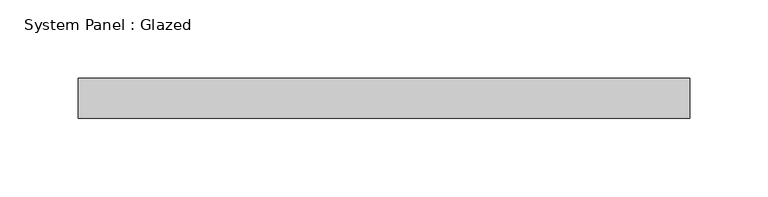
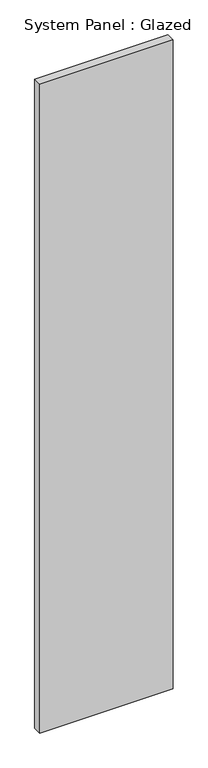
"""IFC4 building model written with IfcOpenShell, lengths in millimetres: plate geometry, System Panel : Glazed."""

from ifc_helpers import new_model, si_unit, origin, origin_with_axes, place, context, project, spatial, polyline, outline, extrude, source, transform, mapped, element, save


def system_panel_glazed_451412b5(model_context):
    return source(origin(), model_context, "Body", "SweptSolid", [
        extrude(outline(polyline([(195.2428622, 19.05), (-195.2428622, 19.05), (-195.2428622, 44.45), (195.2428622, 44.45), (195.2428622, 19.05)])), origin_with_axes(), (0.0, 0.0, 1.0), 2006.6),
    ])


if __name__ == "__main__":
    model = new_model("IFC4")
    model_context = context("Model", 3, world=origin())
    ifc_project = project(units=[si_unit("LENGTHUNIT", "METRE", prefix="MILLI")], contexts=[model_context])
    site = spatial("IfcSite", under=ifc_project)
    building = spatial("IfcBuilding", under=site)
    placement = place(None, origin())
    system_panel_glazed_shape = system_panel_glazed_451412b5(model_context)
    element("IfcPlate", 1, ObjectType="System Panel : Glazed", at=placement, inside=building, context=model_context, shape_type="MappedRepresentation", body=[
        mapped(system_panel_glazed_shape, transform((0.0, 0.0, 0.0), x_axis=(1.0, 0.0, 0.0), y_axis=(0.0, 1.0, 0.0), z_axis=(0.0, 0.0, 1.0))),
    ])
    save(model, "model.ifc")

# Revit data of these elements
# Type "System Panel : Glazed"
#   Construction Type Id = "GSP4R"
#   Analytic Construction = "1/8 in Pilkington single glazing"
#   Visual Light Transmittance = 0.9
#   Solar Heat Gain Coefficient = 0.86
#   Heat Transfer Coefficient (U) = 1.18115 BTU/(h·ft²·°F)
#   Define Thermal Properties by = 1
# Element 1 (IfcPlate, "System Panel : Glazed")
#   Materials on its faces: "Glass"
# Materials
#   "Glass": class "Glass", colour RGB 0 128 192, transparency 0.75, Description = "Soda Lime Glass", Cost = 0
